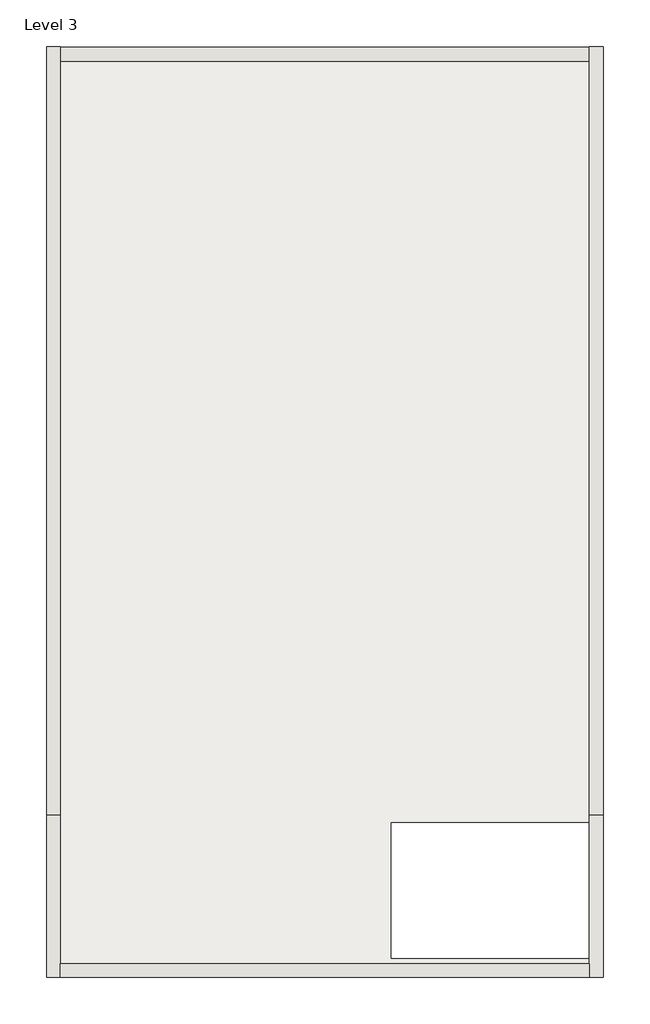
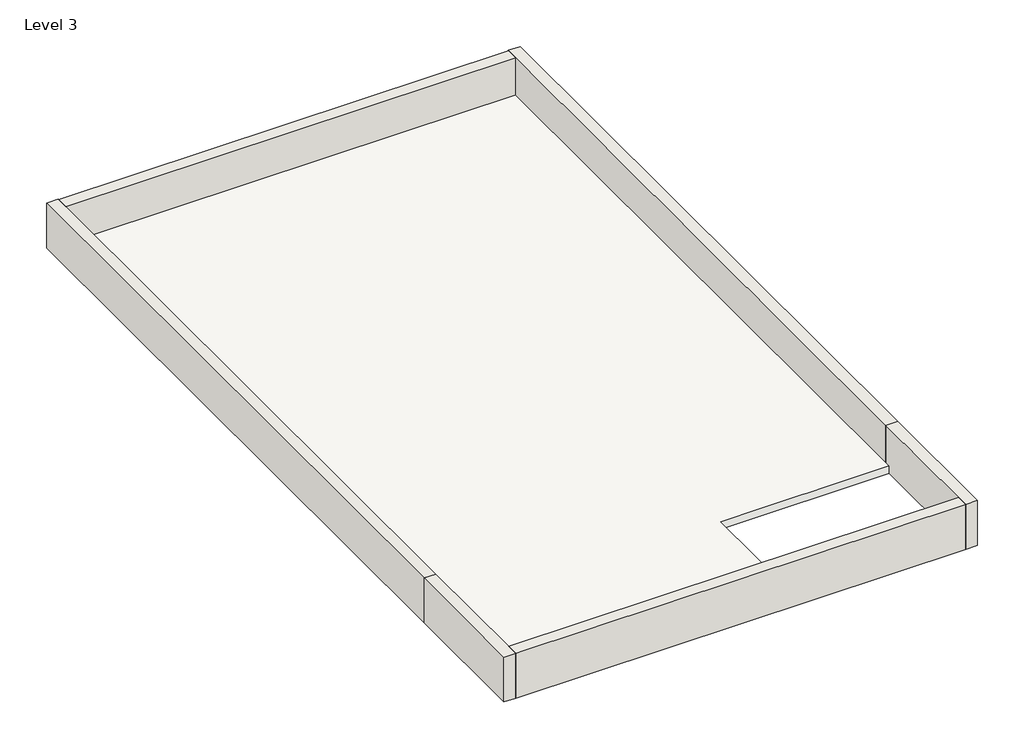
# One storey, incomplete: 6 walls, 1 slab.
"""IFC4 building model written with IfcOpenShell, lengths in millimetres."""

from ifc_helpers import new_model, si_unit, frame, origin, place, context, project, spatial, polyline, outline, extrude, faceted_brep, element, save

model = new_model("IFC4")

# Units and contexts
model_context = context("Model", 3, world=origin())
ifc_project = project(units=[si_unit("LENGTHUNIT", "METRE", prefix="MILLI")], contexts=[model_context])

# Site, building, storey
site = spatial("IfcSite", under=ifc_project)
building = spatial("IfcBuilding", under=site)
storey = spatial("IfcBuildingStorey", under=building, Name="Level 3", Elevation=6248.4)

# Slab
placement = place(None, origin())
element("IfcSlab", 1, ObjectType="6\"", at=placement, inside=storey, context=model_context, shape_type="SweptSolid", body=[
    extrude(outline(polyline([(-1158.4072065, -851.8793133), (-9837.1451282, -851.8793133), (-9837.1451282, 13969.0206867), (-1158.4072065, 13969.0206867), (-1158.4072065, 1472.2206867), (-4412.1017807, 1472.2206867), (-4412.1017807, -776.2596095), (-1158.4072065, -776.2596095), (-1158.4072065, -851.8793133)])), frame((0.0, 0.0, 6248.4), z_axis=(0.0, 0.0, 1.0), x_axis=(1.0, 0.0, 0.0)), (0.0, 0.0, 1.0), 152.4),
])

# Walls
element("IfcWall", 2, ObjectType="9\"", at=placement, inside=storey, context=model_context, shape_type="Brep", body=[
    faceted_brep([(-9837.1451282, -1080.4793133, 6248.4), (-9837.1451282, -851.8793133, 6248.4), (-9837.1451282, 1586.5206867, 6248.4), (-9837.1451282, 1586.5206867, 7162.8), (-9837.1451282, -851.8793133, 7162.8), (-9837.1451282, -1080.4793133, 7162.8), (-10065.7451282, -1080.4793133, 6248.4), (-10065.7451282, -1080.4793133, 7162.8), (-10065.7451282, 1586.5206867, 7162.8), (-10065.7451282, 1586.5206867, 6248.4)], [[[0, 1, 2, 3, 4, 5]], [[6, 7, 8, 9]], [[2, 1, 0, 6, 9]], [[3, 2, 9, 8]], [[5, 4, 3, 8, 7]], [[0, 5, 7, 6]]]),
])
element("IfcWall", 3, ObjectType="9\"", at=placement, inside=storey, context=model_context, shape_type="SweptSolid", body=[
    extrude(outline(polyline([(-9837.1451282, 14197.6206867), (-1150.3451282, 14197.6206867), (-1150.3451282, 13969.0206867), (-9837.1451282, 13969.0206867), (-9837.1451282, 14197.6206867)])), frame((0.0, 0.0, 6248.4), z_axis=(0.0, 0.0, 1.0), x_axis=(1.0, 0.0, 0.0)), (0.0, 0.0, 1.0), 914.4),
])
element("IfcWall", 4, ObjectType="9\"", at=placement, inside=storey, context=model_context, shape_type="SweptSolid", body=[
    extrude(outline(polyline([(-1150.3451282, -1080.4793133), (-9837.1451282, -1080.4793133), (-9837.1451282, -851.8793133), (-1150.3451282, -851.8793133), (-1150.3451282, -1080.4793133)])), frame((0.0, 0.0, 6248.4), z_axis=(0.0, 0.0, 1.0), x_axis=(1.0, 0.0, 0.0)), (0.0, 0.0, 1.0), 914.4),
])
element("IfcWall", 5, ObjectType="9\"", at=placement, inside=storey, context=model_context, shape_type="Brep", body=[
    faceted_brep([(-9837.1451282, 1586.5206867, 6248.4), (-9837.1451282, 13969.0206867, 6248.4), (-9837.1451282, 14197.6206867, 6248.4), (-9837.1451282, 14210.3206867, 6248.4), (-9837.1451282, 14210.3206867, 7162.8), (-9837.1451282, 14197.6206867, 7162.8), (-9837.1451282, 13969.0206867, 7162.8), (-9837.1451282, 1586.5206867, 7162.8), (-10065.7451282, 1586.5206867, 6248.4), (-10065.7451282, 1586.5206867, 7162.8), (-10065.7451282, 14210.3206867, 7162.8), (-10065.7451282, 14210.3206867, 6248.4)], [[[0, 1, 2, 3, 4, 5, 6, 7]], [[8, 9, 10, 11]], [[3, 2, 1, 0, 8, 11]], [[4, 3, 11, 10]], [[7, 6, 5, 4, 10, 9]], [[0, 7, 9, 8]]]),
])
element("IfcWall", 6, ObjectType="9\"", at=placement, inside=storey, context=model_context, shape_type="Brep", body=[
    faceted_brep([(-1150.3451282, 1586.5206867, 6248.4), (-1150.3451282, -851.8793133, 6248.4), (-1150.3451282, -1080.4793133, 6248.4), (-1150.3451282, -1080.4793133, 7162.8), (-1150.3451282, -851.8793133, 7162.8), (-1150.3451282, 1586.5206867, 7162.8), (-921.7451282, 1586.5206867, 6248.4), (-921.7451282, 1586.5206867, 7162.8), (-921.7451282, -1080.4793133, 7162.8), (-921.7451282, -1080.4793133, 6248.4)], [[[0, 1, 2, 3, 4, 5]], [[6, 7, 8, 9]], [[2, 1, 0, 6, 9]], [[5, 4, 3, 8, 7]], [[0, 5, 7, 6]], [[3, 2, 9, 8]]]),
])
element("IfcWall", 7, ObjectType="9\"", at=placement, inside=storey, context=model_context, shape_type="Brep", body=[
    faceted_brep([(-1150.3451282, 14210.3206867, 6248.4), (-1150.3451282, 14197.6206867, 6248.4), (-1150.3451282, 13969.0206867, 6248.4), (-1150.3451282, 1586.5206867, 6248.4), (-1150.3451282, 1586.5206867, 7162.8), (-1150.3451282, 13969.0206867, 7162.8), (-1150.3451282, 14197.6206867, 7162.8), (-1150.3451282, 14210.3206867, 7162.8), (-921.7451282, 14210.3206867, 6248.4), (-921.7451282, 14210.3206867, 7162.8), (-921.7451282, 1586.5206867, 7162.8), (-921.7451282, 1586.5206867, 6248.4)], [[[0, 1, 2, 3, 4, 5, 6, 7]], [[8, 9, 10, 11]], [[3, 2, 1, 0, 8, 11]], [[4, 3, 11, 10]], [[7, 6, 5, 4, 10, 9]], [[0, 7, 9, 8]]]),
])

save(model, "model.ifc")

# Revit data of these elements
# Type "6\""
#   Assembly Code = "B1010"
#   Function = 0
#   Layers, outside or top first: 0' - 6" "FLOORING" (function 1)
# Type "9\""
#   Assembly Code = "B2010"
#   Layers, outside or top first: 0' - 9" "ext walls" (function 1)
# Element 1 (IfcSlab, "6\"")
#   Height Offset From Level = 0' - 6"
#   Phase Created = New Construction
#   Materials on its faces: "FLOORING"
# Elements 2, 3, 4, 5, 6, 7 (IfcWall, "9\"")
#   Top Offset = 0' - 0"
#   Base Offset = 0' - 0"
#   Unconnected Height = 3' - 0"
#   wall height = 3' - 0"
#   Phase Created = New Construction
#   Base Constraint = Level 3
#   Materials on its faces: "ext walls"
# Materials
#   "FLOORING": class "Generic", colour RGB 124 103 75, transparency 0, Cost = 0
#   "ext walls": class "Generic", colour RGB 120 120 120, transparency 0, Cost = 0
